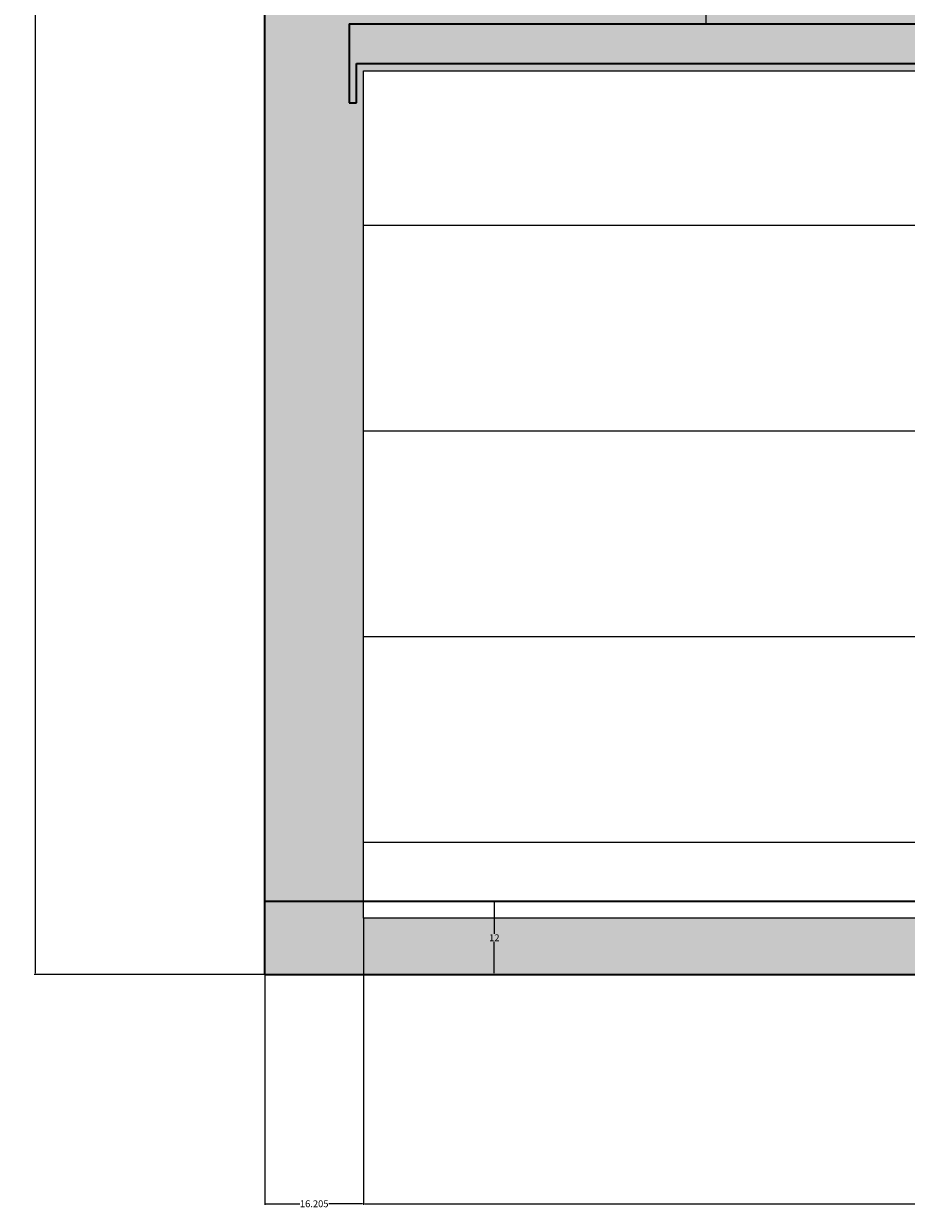
# Model space of a CAD drawing. Units: inches. Extents: x 8 to 634, y 41 to 867.
# Tile 1 of 21: x 8 to 153, y 41 to 236. Entities that reach past the tile are written whole.
import ezdxf

# ---------------------------------------------------------------- set-up
doc = ezdxf.new("R2010")
doc.units = ezdxf.units.IN
doc.header["$MEASUREMENT"] = 0
for name, color, linetype, lineweight in [('A-ANNO-DIMS', 2, 'Continuous', 18), ('A-DOOR', 3, 'Continuous', 25), ('A-DOOR-PATT', 8, 'Continuous', 9), ('A-FLOR', 7, 'Continuous', 35), ('A-FLOR-PATT', 8, 'Continuous', 9), ('A-WALL', 7, 'Continuous', 35), ('A-WALL-PANL', 7, 'Continuous', 18), ('A-WALL-PATT', 8, 'Continuous', 9)]:
    doc.layers.add(name, color=color, linetype=linetype, lineweight=lineweight)
doc.styles.get("Standard").update_dxf_attribs({"font": 'arial.ttf'})
doc.dimstyles.get("Standard").update_dxf_attribs({"dimtxt": 1.125, "dimasz": 0.18, "dimexe": 0.18, "dimexo": 0.0625, "dimgap": 0.09, "dimtad": 0, "dimtih": 1, "dimtoh": 1, "dimdec": 4, "dimzin": 0, "dimdsep": 46, "dimlunit": 4, "dimtxsty": 'Standard', "dimcen": 0.09, "dimadec": 0, "dimazin": 0, "dimtfac": 1, "dimtdec": 4, "dimtofl": 0, "dimtmove": 0, "dimatfit": 3, "dimfxl": 1, "dimtolj": 1, "dimtzin": 0, "dimarcsym": 0})

# ---------------------------------------------------------------- blocks, each defined once
blk = doc.blocks.new('*D20')
at = {"layer": 'A-ANNO-DIMS', "color": 0, "lineweight": -2, "transparency": 16777216}
for p, q in [((144.29, 828.98), (9.51, 828.98)), ((9.69, 828.8), (9.69, 454.93)), ((9.69, 79.74), (9.69, 453.6)), ((47.28, 79.56), (9.51, 79.56))]:
    blk.add_line(p, q, dxfattribs=at)
at = {"layer": 'A-ANNO-DIMS', "color": 0, "transparency": 16777216}
for points in [[(9.66, 828.8), (9.72, 828.8), (9.69, 828.98)], [(9.66, 79.74), (9.72, 79.74), (9.69, 79.56)]]:
    blk.add_solid(points, dxfattribs=at)
at = {"layer": 'Defpoints', "color": 0, "transparency": 16777216}
for p in [(9.69, 828.98), (144.36, 828.98), (47.34, 79.56)]:
    blk.add_point(p, dxfattribs=at)
at = {"layer": 'A-ANNO-DIMS', "color": 0, "transparency": 16777216, "insert": (9.69, 454.27), "char_height": 1.125, "attachment_point": 5}
blk.add_mtext('\\A1;749.4', dxfattribs=at)
blk = doc.blocks.new('*D28')
at = {"layer": 'A-ANNO-DIMS', "color": 0, "lineweight": -2, "transparency": 16777216}
for p, q in [((47.34, 91.49), (47.34, 41.73)), ((63.54, 88.73), (63.54, 41.73)), ((47.52, 41.91), (53.07, 41.91)), ((63.36, 41.91), (57.82, 41.91))]:
    blk.add_line(p, q, dxfattribs=at)
at = {"layer": 'A-ANNO-DIMS', "color": 0, "transparency": 16777216}
for points in [[(47.52, 41.94), (47.52, 41.88), (47.34, 41.91)], [(63.36, 41.94), (63.36, 41.88), (63.54, 41.91)]]:
    blk.add_solid(points, dxfattribs=at)
at = {"layer": 'Defpoints', "color": 0, "transparency": 16777216}
for p in [(47.34, 91.56), (63.54, 88.79), (63.54, 41.91)]:
    blk.add_point(p, dxfattribs=at)
at = {"layer": 'A-ANNO-DIMS', "color": 0, "transparency": 16777216, "insert": (55.44, 41.91), "char_height": 1.125, "attachment_point": 5}
blk.add_mtext('\\A1;16.205', dxfattribs=at)
blk = doc.blocks.new('*D29')
at = {"layer": 'A-ANNO-DIMS', "color": 0, "lineweight": -2, "transparency": 16777216}
for p, q in [((63.54, 88.73), (63.54, 41.73)), ((269, 88.73), (269, 41.73)), ((63.72, 41.91), (163.83, 41.91)), ((268.82, 41.91), (168.71, 41.91))]:
    blk.add_line(p, q, dxfattribs=at)
at = {"layer": 'A-ANNO-DIMS', "color": 0, "transparency": 16777216}
for points in [[(63.72, 41.94), (63.72, 41.88), (63.54, 41.91)], [(268.82, 41.94), (268.82, 41.88), (269, 41.91)]]:
    blk.add_solid(points, dxfattribs=at)
at = {"layer": 'Defpoints', "color": 0, "transparency": 16777216}
for p in [(63.54, 88.79), (269, 88.79), (269, 41.91)]:
    blk.add_point(p, dxfattribs=at)
at = {"layer": 'A-ANNO-DIMS', "color": 0, "transparency": 16777216, "insert": (166.27, 41.91), "char_height": 1.125, "attachment_point": 5}
blk.add_mtext('\\A1;205.45', dxfattribs=at)
blk = doc.blocks.new('*D61')
at = {"layer": 'A-ANNO-DIMS', "color": 0, "lineweight": -2, "transparency": 16777216}
for p, q in [((47.4, 91.56), (85.17, 91.56)), ((84.99, 91.38), (84.99, 86.21)), ((84.99, 79.74), (84.99, 84.9)), ((47.4, 79.56), (85.17, 79.56))]:
    blk.add_line(p, q, dxfattribs=at)
at = {"layer": 'A-ANNO-DIMS', "color": 0, "transparency": 16777216}
for points in [[(84.96, 91.38), (85.02, 91.38), (84.99, 91.56)], [(84.96, 79.74), (85.02, 79.74), (84.99, 79.56)]]:
    blk.add_solid(points, dxfattribs=at)
at = {"layer": 'Defpoints', "color": 0, "transparency": 16777216}
for p in [(47.34, 91.56), (47.34, 79.56), (84.99, 79.56)]:
    blk.add_point(p, dxfattribs=at)
at = {"layer": 'A-ANNO-DIMS', "color": 0, "transparency": 16777216, "insert": (84.99, 85.56), "char_height": 1.125, "attachment_point": 5}
blk.add_mtext('\\A1;12', dxfattribs=at)

msp = doc.modelspace()

# ---------------------------------------------------------------- hatches: boundary and pattern name
at = {"layer": 'A-DOOR-PATT', "transparency": 33554687}
h = msp.add_hatch(dxfattribs=at)
h.set_pattern_fill('ANSI31', color=256, scale=270, angle=135)
h.paths.add_polyline_path([(268.998, 227.8036), (63.5448, 227.8036), (63.5448, 91.5555), (268.998, 91.5555)])
at = {"layer": 'A-FLOR-PATT', "transparency": 33554687}
h = msp.add_hatch(dxfattribs=at)
h.set_pattern_fill('AR-CONC', color=256, scale=0.76, angle=135)
h.set_pattern_definition([(185, (0, 0), (-3.517334, 4.191795), [0.57, -6.27]), (130, (0, 0), (-3.29664, -4.78794), [0.456, -5.016]), (235.4514, (-0.293, 0.3493), (-6.81397, -0.596145), [0.484425, -5.32868]), (181.1842, (-1.075, -1.075), (-4.845865, 6.62487), [0.855, -9.405]), (231.6356, (-1.479, -0.523), (-10.25781, -0.21204), [0.72664, -7.99302]), (126.1842, (-1.075, -1.075), (-10.25781, -0.21204), [0.684, -7.524]), (156, (-1.3435, -0.2687), (-1.044107, 5.371464), [0.57, -6.27]), (101, (-1.3435, -0.2687), (-5.204544, -2.589385), [0.456, -5.016]), (206.4514, (-1.4305, 0.179), (-6.24865, 2.78208), [0.484425, -5.32868]), (172.5, (0, 0), (-1.8543226, -1.723628), [0, -4.9552, 0, -5.092, 0, -5.035]), (142.5, (0, 0), (-3.533312, -0.705834), [0, -2.9032, 0, -4.8412, 0, -1.919]), (102.5, (1.1984, -1.1984), (-2.747558, 2.989978), [0, -1.9, 0, -5.928, 0, -7.866]), (92.5, (1.7358, -1.7358), (-3.672015, 2.596084), [0, -2.47, 0, -3.9368, 0, -5.586])])
h.paths.add_polyline_path([(594.3501, 91.5417), (360.785, 91.5417), (295.0049, 91.5417), (268.998, 91.5432), (268.998, 88.7912), (63.5448, 88.7912), (63.5448, 91.5555), (47.3401, 91.5555), (47.3401, 79.5555), (349.489, 79.5555), (594.3501, 79.5555)])
at = {"layer": 'A-WALL-PATT', "transparency": 33554687}
h = msp.add_hatch(dxfattribs=at)
h.set_pattern_fill('AR-CONC', color=256, scale=3.2)
h.paths.add_polyline_path([(119.7065, 697.6655), (47.3401, 697.6655), (47.3401, 569.1705), (119.7065, 569.1705)])
h.paths.add_polyline_path([(202.1558, 697.6655), (119.7065, 697.6655), (119.7065, 569.1705), (202.1558, 569.1705)])
h.paths.add_polyline_path([(284.6051, 697.6655), (202.1558, 697.6655), (202.1558, 569.1705), (284.6051, 569.1705)])
h.paths.add_polyline_path([(119.7065, 569.1705), (47.3401, 569.1705), (47.3401, 523.5555), (47.3401, 449.7533), (119.7065, 449.7533)])
h.paths.add_polyline_path([(342.6544, 682.1444), (360.785, 697.6655), (284.6051, 697.6655), (284.6051, 569.1705), (342.6544, 569.1705)])
h.paths.add_polyline_path([(342.6544, 569.1705), (284.6051, 569.1705), (284.6051, 449.7533), (342.6544, 449.7533)])
h.paths.add_polyline_path([(418.2881, 691.978), (418.2881, 697.6655), (360.785, 697.6655), (360.785, 569.1705), (418.2881, 569.1705)])
h.paths.add_polyline_path([(418.2881, 569.1705), (360.785, 569.1705), (360.785, 523.5555), (360.785, 449.7533), (418.2881, 449.7533)])
h.paths.add_polyline_path([(594.3501, 697.6655), (539.0002, 697.6655), (539.0002, 691.978), (539.0002, 569.1705), (594.3501, 569.1705)])
h.paths.add_polyline_path([(594.3501, 523.5555), (594.3501, 569.1705), (539.0002, 569.1705), (539.0002, 451.6305), (594.3501, 451.6305)])
h.paths.add_polyline_path([(594.3501, 451.6305), (539.0002, 451.6305), (539.0002, 391.7598), (594.3501, 391.7598)])
h.paths.add_polyline_path([(594.3501, 391.7598), (539.0002, 391.7598), (539.0002, 276.166), (594.3501, 276.166)])
h.paths.add_polyline_path([(418.2881, 449.7533), (360.785, 449.7533), (360.785, 391.7598), (418.2881, 391.7598)])
h.paths.add_polyline_path([(342.6544, 449.7533), (284.6051, 449.7533), (284.6051, 391.7598), (342.6544, 391.7598)])
h.paths.add_polyline_path([(342.6544, 391.7598), (284.6051, 391.7598), (284.6051, 272.3426), (342.6544, 272.3426)])
h.paths.add_polyline_path([(418.2881, 391.7598), (360.785, 391.7598), (360.785, 272.3426), (418.2881, 272.3426)])
h.paths.add_polyline_path([(418.2881, 272.3426), (360.785, 272.3426), (360.785, 235.5555), (418.2881, 235.5555)])
h.paths.add_polyline_path([(342.6544, 272.3426), (284.6051, 272.3426), (284.6051, 235.5555), (295.0049, 235.5555), (342.6544, 235.5555)])
h.paths.add_polyline_path([(594.3501, 276.166), (539.0002, 276.166), (539.0002, 228.4951), (594.3501, 228.4951)])
h.paths.add_polyline_path([(594.3501, 228.4951), (539.0002, 228.4951), (539.0002, 91.5417), (594.3501, 91.5417)])
h.paths.add_polyline_path([(418.2881, 235.5555), (360.785, 235.5555), (360.785, 91.5417), (418.2881, 91.5417)])
h.paths.add_polyline_path([(284.6051, 272.3426), (119.7065, 272.3426), (119.7065, 235.5555), (284.6051, 235.5555)])
h.paths.add_polyline_path([(119.7065, 272.3426), (47.3401, 272.3426), (47.3401, 235.5555), (47.3401, 91.5555), (63.5448, 91.5555), (63.5448, 227.8036), (268.998, 227.8036), (268.998, 91.5555), (295.0049, 91.5555), (295.0049, 222.583), (271.9787, 222.583), (271.9787, 229.0481), (62.4019, 229.0481), (62.4019, 222.583), (61.1827, 222.583), (61.1827, 235.5555), (119.7065, 235.5555)])
h.paths.add_polyline_path([(119.7065, 391.7598), (47.3401, 391.7598), (47.3401, 379.5555), (47.3401, 272.3426), (119.7065, 272.3426)])
h.paths.add_polyline_path([(119.7065, 449.7533), (47.3401, 449.7533), (47.3401, 391.7598), (119.7065, 391.7598)])
h.paths.add_polyline_path([(202.1558, 449.7533), (119.7065, 449.7533), (119.7065, 391.7598), (202.1558, 391.7598)])
h.paths.add_polyline_path([(284.6051, 449.7533), (202.1558, 449.7533), (202.1558, 391.7598), (284.6051, 391.7598)])
at = {"layer": 'A-WALL-PATT', "transparency": 33554554}
h = msp.add_hatch(dxfattribs=at)
h.set_pattern_fill('AR-CONC', color=256, scale=0.76, angle=135)
h.paths.add_polyline_path([(295.0049, 235.5555), (61.1827, 235.5555), (61.1827, 222.583), (62.4019, 222.583), (62.4019, 229.0481), (271.9787, 229.0481), (271.9787, 222.583), (295.0049, 222.583)])

# ---------------------------------------------------------------- linework, layer by layer
at = {"layer": 'A-DOOR'}
msp.add_lwpolyline([(63.5448, 227.8036), (268.998, 227.8036), (268.998, 88.7912), (63.5448, 88.7912)], close=True, dxfattribs=at)
at = {"layer": 'A-FLOR'}
for p, q in [((47.3401, 79.5555), (47.3401, 91.5555)), ((47.3401, 91.5555), (349.489, 91.5555)), ((47.3401, 79.5555), (349.489, 79.5555))]:
    msp.add_line(p, q, dxfattribs=at)
at = {"layer": 'A-WALL'}
for p, q in [((47.3401, 235.5555), (47.3401, 379.5555)), ((47.3401, 91.5555), (47.3401, 235.5555)), ((61.1827, 235.5555), (61.1827, 222.583)), ((61.1827, 235.5555), (295.0049, 235.5555)), ((62.4019, 222.583), (62.4019, 229.0481)), ((62.4019, 229.0481), (271.9787, 229.0481)), ((61.1827, 222.583), (62.4019, 222.583))]:
    msp.add_line(p, q, dxfattribs=at)
at = {"layer": 'A-WALL-PANL'}
msp.add_line((119.7065, 272.3426), (119.7065, 235.5555), dxfattribs=at)

# ---------------------------------------------------------------- dimensions: what is measured, and where the dimension line sits
at = {"layer": 'A-ANNO-DIMS'}
for base, p1, p2, angle, override, picture, middle in [((9.6901, 828.9821), (47.3401, 79.5555), (144.3564, 828.9821), 90, {"dimdec": 1, "dimlfac": 1, "dimrnd": 0, "dimzin": 0, "dimdsep": 46, "dimlunit": 2}, '*D20', (9.6901, 454.2688)), ((84.9901, 79.5555), (47.3401, 91.5555), (47.3401, 79.5555), 270, {"dimdec": 0, "dimlfac": 1, "dimrnd": 0, "dimzin": 0, "dimdsep": 46, "dimlunit": 2}, '*D61', (84.9901, 85.5555))]:
    dim = msp.add_linear_dim(base=base, p1=p1, p2=p2, angle=angle, dimstyle='Standard', override=override, dxfattribs=at)
    dim.commit()
    dim.dimension.update_dxf_attribs({"geometry": picture, "text_midpoint": middle})
for base, p1, p2, override, picture, middle in [((63.5448, 41.9055), (47.3401, 91.5555), (63.5448, 88.7912), {"dimdec": 3, "dimlfac": 1, "dimrnd": 0, "dimzin": 0, "dimdsep": 46, "dimlunit": 2}, '*D28', (55.4425, 41.9055)), ((268.998, 41.9055), (63.5448, 88.7912), (268.998, 88.7912), {"dimdec": 2, "dimlfac": 1, "dimrnd": 0, "dimzin": 0, "dimdsep": 46, "dimlunit": 2}, '*D29', (166.2714, 41.9055))]:
    dim = msp.add_linear_dim(base=base, p1=p1, p2=p2, dimstyle='Standard', override=override, dxfattribs=at)
    dim.commit()
    dim.dimension.update_dxf_attribs({"geometry": picture, "text_midpoint": middle})

doc.saveas('drawing.dxf')
